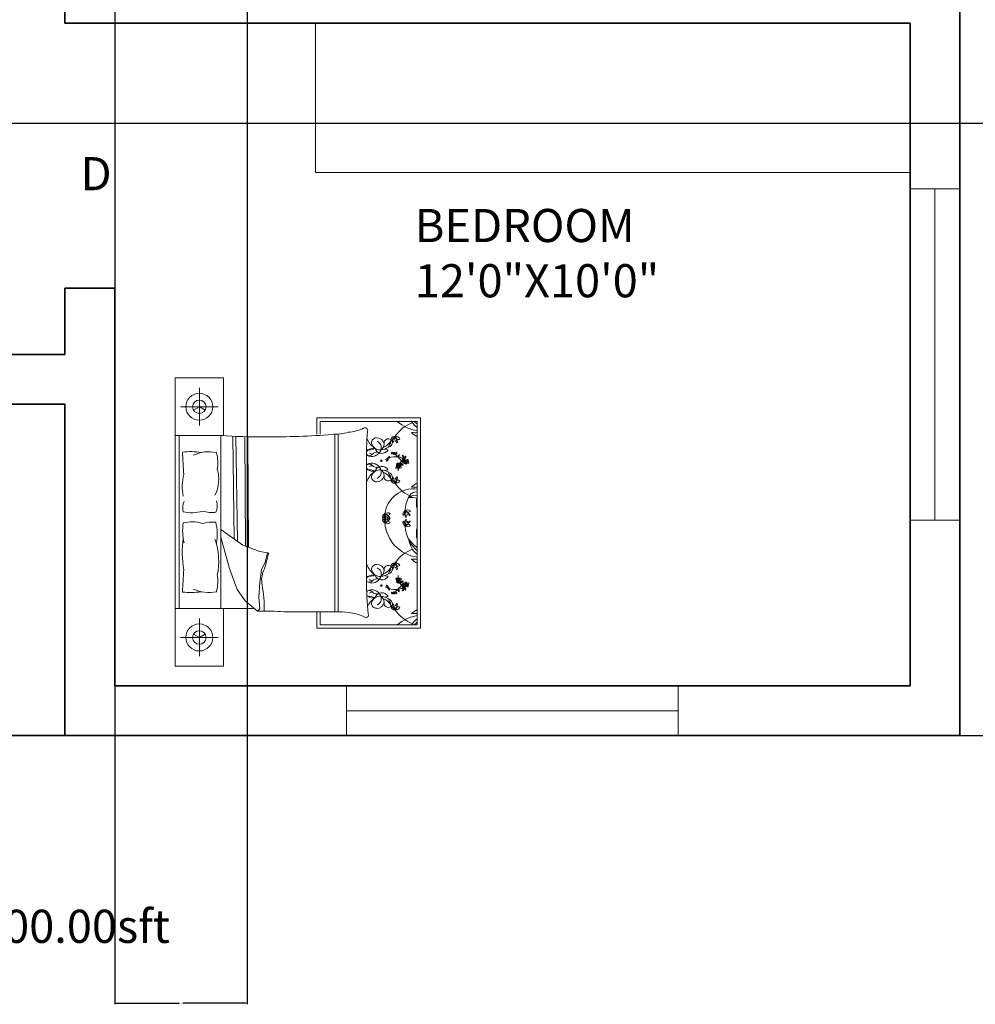
# Model space of a CAD drawing. Units: inches. Extents: x -43 to 1296, y -568 to 542.
# Tile 9 of 14: x 1014 to 1187, y -532 to -354. Entities that reach past the tile are written whole.
import ezdxf

# ---------------------------------------------------------------- set-up
doc = ezdxf.new("R2010")
doc.units = ezdxf.units.IN
doc.header["$MEASUREMENT"] = 0
for name, color, linetype, lineweight in [('A-ANNO-DIMS', 2, 'Continuous', 18), ('A-ANNO-SYMB', 7, 'Continuous', 25), ('A-ANNO-TEXT', 7, 'Continuous', 18), ('A-AREA-IDEN', 7, 'Continuous', 18), ('A-FLOR-CASE', 9, 'Continuous', 18), ('A-FURN', 8, 'Continuous', 13), ('A-GLAZ', 6, 'Continuous', 18), ('A-WALL', 7, 'Continuous', 35)]:
    doc.layers.add(name, color=color, linetype=linetype, lineweight=lineweight)
doc.styles.get("Standard").update_dxf_attribs({"font": 'arial.ttf'})
doc.dimstyles.get("Standard").update_dxf_attribs({"dimtxt": 0.18, "dimasz": 0.18, "dimexe": 0.18, "dimexo": 0.0625, "dimgap": 0.09, "dimtad": 0, "dimtih": 1, "dimtoh": 1, "dimdec": 0, "dimzin": 0, "dimdsep": 46, "dimlunit": 3, "dimtxsty": 'Standard', "dimcen": 0.09, "dimadec": 0, "dimazin": 0, "dimtfac": 1, "dimtdec": 0, "dimtofl": 0, "dimtmove": 0, "dimatfit": 3, "dimfxl": 1, "dimtolj": 1, "dimtzin": 0, "dimarcsym": 0})

# ---------------------------------------------------------------- blocks, each defined once
blk = doc.blocks.new('*D4')
at = {"layer": 'A-ANNO-DIMS', "color": 0, "lineweight": -2, "transparency": 16777216}
for p, q in [((1184.19, -3.76), (1201.25, -3.76)), ((1201.07, -3.94), (1201.07, -240.61)), ((1201.07, -483.58), (1201.07, -246.91)), ((1184.19, -483.76), (1201.25, -483.76))]:
    blk.add_line(p, q, dxfattribs=at)
at = {"layer": 'A-ANNO-DIMS', "color": 0, "transparency": 16777216}
for points in [[(1201.04, -3.94), (1201.1, -3.94), (1201.07, -3.76)], [(1201.04, -483.58), (1201.1, -483.58), (1201.07, -483.76)]]:
    blk.add_solid(points, dxfattribs=at)
at = {"layer": 'Defpoints', "color": 0, "transparency": 16777216}
for p in [(1184.13, -3.76), (1184.13, -483.76), (1201.07, -483.76)]:
    blk.add_point(p, dxfattribs=at)
at = {"layer": 'A-ANNO-DIMS', "color": 0, "transparency": 16777216, "insert": (1201.07, -243.76), "char_height": 6, "attachment_point": 5}
blk.add_mtext("\\A1;40'", dxfattribs=at)
blk = doc.blocks.new('BED-SUITE-52')
for p, q in [((0, 0), (0, 52.23)), ((4.35, 43.59), (4.35, 50.42)), ((7.76, 47), (0.94, 47)), ((25.6, 42.07), (25.6, 44.97)), ((25.6, 44.97), (44.41, 44.97)), ((44.41, 44.97), (44.41, 6.89)), ((26.21, 44.36), (26.21, 42.06)), ((43.81, 44.36), (26.21, 44.36)), ((43.81, 7.5), (43.81, 44.36)), ((0.67, 41.78), (0.67, 10.45)), ((8.25, 10.45), (8.25, 41.78)), ((10.42, 41.64), (10.68, 23.05)), ((10.96, 41.62), (11.23, 22.66)), ((12.6, 41.59), (12.68, 21.76)), ((13.14, 41.6), (13.22, 21.56)), ((28.86, 42.02), (28.86, 9.84)), ((29.51, 42.07), (29.51, 9.84)), ((38.51, 39.22), (37.92, 39.33)), ((34.64, 36.72), (34.64, 15.51)), ((38.51, 35.57), (37.92, 35.45)), ((8.25, 24.79), (12.24, 21.93)), ((9.81, 17.7), (8.25, 23.4)), ((12.24, 21.93), (15.3, 20.77)), ((15.3, 20.77), (16.68, 20.56)), ((16.68, 20.56), (16.25, 18.86)), ((16.25, 18.86), (15.62, 17.49)), ((11.18, 13.89), (9.81, 17.7)), ((15.62, 17.49), (15.3, 15.16)), ((38.51, 16.3), (37.92, 16.41)), ((15.3, 15.16), (15.09, 12.52)), ((12.66, 11.88), (11.18, 13.89)), ((15.09, 12.52), (15.3, 10.4)), ((38.51, 12.65), (37.92, 12.53)), ((14.88, 9.98), (12.66, 11.88)), ((0, 10.45), (14.33, 10.45)), ((15.3, 10.4), (14.88, 9.98)), ((25.6, 6.89), (25.6, 9.85)), ((26.21, 9.85), (26.21, 7.5)), ((4.35, 8.64), (4.35, 1.81)), ((26.21, 7.5), (43.81, 7.5)), ((44.41, 6.89), (25.6, 6.89)), ((7.76, 5.22), (0.94, 5.22))]:
    blk.add_line(p, q)
for points in [[(0, 41.78), (8.7, 41.78), (8.7, 52.23), (0, 52.23)], [(4.35, 47), (3.3, 46.39)], [(4.35, 47), (5.41, 46.39)], [(8.7, 10.45), (8.7, 0), (0, 0)], [(4.35, 5.22), (3.3, 5.83)], [(4.35, 5.22), (5.41, 5.83)]]:
    blk.add_lwpolyline(points)
for points in [[(28.45, 42, 0.056112), (31.32, 42.38, 0.095341), (34.09, 43.12)], [(1.3, 38.78, -0.074897), (4.71, 38.72, 0.472817)], [(4.9, 28.1, -0.14099), (1.42, 27.99, -0.235245)], [(4.9, 25.87, 0.14099), (1.42, 25.97, 0.235245)], [(1.3, 13.45, 0.074897), (4.71, 13.51, -0.472817)], [(19.66, 9.87, 0.001242), (29.57, 9.84, -0.127202), (34.51, 8.8)]]:
    blk.add_lwpolyline(points, format="xyb")
for centre, radius in [((4.35, 47), 2.44), ((4.35, 47), 1.22), ((40.41, 36.2), 0.133), ((41.81, 37.07), 0.133), ((40.41, 15.66), 0.133), ((41.81, 14.79), 0.133), ((4.35, 5.22), 2.44), ((4.35, 5.22), 1.22)]:
    blk.add_circle(centre, radius)
for centre, radius, start, end in [((34.35, 42.72), 0.476, 336.5219, 123.8264), ((45.4, 37.77), 6.82, 111.4092, 145.6135), ((44.73, 49.44), 6.82, 228.1144, 262.255), ((45.64, 46.02), 3.32, 209.8884, 236.5383), ((46.26, 47.22), 4.14, 223.5186, 233.6964), ((14.64, 135.41), 93.84, 266.1, 270.9282), ((18.05, 163.97), 122.41, 269.1145, 274.8735), ((85.43, 38.32), 50.82, 175.2402, 181.8035), ((38.32, 42.79), 3.95, 203.6453, 236.3329), ((36.42, 40.49), 0.882, 88.9462, 185.5144), ((36.55, 40.12), 1.25, 7.1143, 95.0551), ((38.56, 40.41), 0.784, 19.1312, 189.736), ((39.64, 41.08), 0.565, 76.272, 177.0484), ((38.78, 42.23), 1.16, 284.7031, 328.6173), ((40.4, 40.75), 1.08, 125.7657, 194.5347), ((35.12, 42.66), 4.77, 332.8176, 347.4827), ((39.94, 40.89), 0.756, 20.9613, 102.2885), ((40.34, 41.64), 0.57, 181.7131, 301.5367), ((38.48, 40.49), 1.72, 2.0648, 41.1598), ((39.52, 41.13), 0.558, 316.2238, 62.3173), ((44.87, 44.16), 2.77, 221.0454, 247.4453), ((43.38, 51.75), 9.44, 266.3481, 272.5919), ((35.03, 41.34), 2.16, 259.249, 301.1782), ((35.97, 37.49), 2.01, 85.2696, 124.215), ((37.07, 40.76), 1.57, 193.079, 274.7067), ((37.39, 39.86), 1.3, 196.8663, 330.0915), ((36.07, 39.63), 1.21, 338.5779, 68.4181), ((36.27, 40.34), 1.52, 305.9599, 357.6409), ((37.03, 41.99), 2.8, 273.4924, 303.7117), ((36.83, 41.97), 2.47, 288.2955, 328.7386), ((38.32, 40.6), 0.979, 285.6955, 4.031), ((39.62, 39.55), 1.04, 128.4175, 173.8338), ((39.41, 40.57), 0.48, 126.7319, 206.0245), ((39.84, 40.8), 0.0445, 20.2667, 316.2271), ((40.07, 40.56), 0.0411, 52.0591, 168.5166), ((40.11, 40.55), 0.0847, 168.5166, 2.0648), ((-495.72, 9.99), 497.85, 2.8502, 3.3148), ((6.08, 32.13), 6.73, 78.2417, 114.8684), ((0.69, 36.92), 7, 348.9631, 14.8961), ((35.22, 38.66), 0.629, 196.6343, 225.5483), ((35.22, 38.66), 0.629, 127.675, 162.5814), ((35.59, 39.66), 1.66, 240.8249, 340.7178), ((35.09, 38.92), 0.781, 246.1646, 318.4347), ((35.89, 39.91), 1.5, 240.0851, 262.564), ((36.48, 37.7), 1.07, 74.8529, 138.4347), ((36.84, 39.04), 0.324, 254.8529, 12.6959), ((35.97, 37.49), 2.01, 53.6555, 57.2989), ((39.96, 33.62), 4.33, 110.1059, 116.9968), ((37.57, 37.74), 0.839, 336.3901, 344.4871), ((38.48, 37.52), 0.106, 83.9457, 185.6216), ((38.06, 37.62), 0.438, 328.836, 0.8141), ((38.28, 37.49), 0.251, 306.5232, 32.4668), ((38.58, 37.69), 0.106, 112.5583, 214.2343), ((38.51, 37.88), 0.251, 265.7131, 351.6568), ((38.29, 38.02), 0.438, 297.3659, 329.344), ((37.96, 38.39), 0.839, 313.6929, 321.7899), ((38.89, 37.82), 0.274, 115.5379, 168.6744), ((37.96, 38.21), 0.825, 329.344, 349.7412), ((39.96, 33.62), 4.33, 86.1723, 106.4158), ((37.3, 38.02), 1.47, 352.8698, 1.6736), ((39.25, 38.55), 0.103, 125.0752, 284.7644), ((39.41, 38.59), 0.222, 127.3642, 168.4363), ((39.24, 38.77), 0.32, 277.4968, 341.2737), ((39.49, 38.62), 0.127, 88.1325, 178.8919), ((39.75, 38.49), 0.275, 136.3462, 189.6513), ((39.62, 38.78), 0.133, 183.2768, 356.7232), ((39.59, 38.46), 0.115, 189.6513, 312.3208), ((40.03, 38.54), 0.435, 164.2829, 186.9148), ((39.52, 38.54), 0.218, 312.3208, 40.2111), ((39.98, 38.78), 0.309, 201.6382, 274.947), ((39.57, 38.36), 0.404, 42.3896, 66.5724), ((43.64, 41.56), 4.96, 217.9541, 226.8459), ((39.86, 38.6), 0.22, 10.9597, 52.2379), ((40, 38.58), 0.102, 274.947, 37.5263), ((40.34, 38), 0.106, 112.5583, 214.2343), ((40.27, 38.19), 0.251, 265.7131, 351.6568), ((40.05, 38.33), 0.438, 297.3659, 329.344), ((40.07, 35.78), 2.17, 60.7959, 85.244), ((35.46, 32.66), 7.14, 37.8256, 47.7588), ((39.72, 38.7), 0.839, 313.6929, 321.7899), ((40.65, 38.13), 0.274, 115.5379, 168.6744), ((39.72, 38.52), 0.825, 329.344, 349.7412), ((39.06, 38.33), 1.47, 352.8698, 1.6736), ((42.95, 35.55), 2.6, 130.182, 149.456), ((41.13, 38.04), 0.148, 33.0979, 123.1364), ((37.86, 35.94), 3.89, 31.1156, 34.8118), ((40.91, 37.78), 0.402, 2.3172, 70.5201), ((40.72, 37.35), 0.606, 310.9365, 22.7695), ((41.25, 37.68), 0.116, 135.7354, 318.1297), ((41.05, 37.87), 0.154, 315.7354, 31.1156), ((40.92, 37.55), 0.357, 319.3812, 5.5456), ((41.33, 37.68), 0.116, 68.2452, 250.6395), ((41.07, 37.83), 0.346, 352.6008, 57.1845), ((42.3, 35.5), 2.32, 111.7087, 116.2181), ((41.4, 37.91), 0.346, 252.8042, 349.6943), ((41.07, 37.29), 0.369, 331.1838, 51.6792), ((40.07, 35.78), 2.17, 47.5083, 55.9967), ((41.43, 37.93), 0.154, 248.2452, 323.6254), ((41.3, 38.03), 0.402, 291.7087, 3.0299), ((38.43, 40.15), 3.89, 323.6254, 327.3216), ((41.61, 37.93), 0.148, 325.6077, 55.6462), ((42.21, 37.11), 0.419, 121.9501, 165.2442), ((42.06, 37.35), 0.132, 44.3732, 121.9501), ((1.21, 33.9), 6.65, 333.8761, 16.1746), ((35.22, 36.13), 0.629, 134.4517, 156.7144), ((35.22, 36.13), 0.629, 203.2856, 232.325), ((35.59, 35.12), 1.66, 19.2822, 119.1751), ((35.09, 35.86), 0.781, 41.5653, 113.8354), ((35.89, 34.87), 1.5, 97.436, 119.9149), ((36.48, 37.09), 1.07, 221.5653, 285.1471), ((37.39, 34.92), 1.3, 29.9085, 163.1337), ((36.84, 35.74), 0.324, 347.3041, 105.1471), ((35.97, 37.29), 2.01, 302.7011, 306.3445), ((37.27, 37.25), 0.164, 169.5864, 349.5616), ((36.27, 34.44), 1.52, 2.3591, 54.0401), ((37.33, 37.24), 0.101, 349.5616, 167.2949), ((38.51, 37.19), 0.274, 129.5056, 182.6421), ((37.73, 37.82), 0.825, 308.4388, 328.836), ((37.58, 38.49), 1.47, 296.5064, 305.3102), ((40.04, 35.98), 0.103, 125.0752, 284.7644), ((40.2, 36.02), 0.222, 93.635, 168.4363), ((40.21, 37.22), 0.606, 253.6301, 325.4631), ((40.38, 36.38), 0.429, 82.0748, 142.6895), ((40.33, 36.97), 0.441, 228.342, 274.9894), ((40.17, 36.37), 0.13, 138.2946, 276.2474), ((40.03, 36.19), 0.32, 277.4968, 341.2737), ((40.22, 36.35), 0.181, 358.5719, 143.8954), ((40.28, 36.04), 0.127, 88.1325, 178.8919), ((40.33, 36.49), 0.183, 208.8493, 269.9355), ((40.17, 36.45), 0.209, 274.2123, 318.1587), ((40.54, 35.91), 0.275, 136.3462, 189.6513), ((40.38, 35.88), 0.115, 189.6513, 312.3208), ((42.95, 35.55), 2.6, 175.2415, 182.8929), ((40.34, 36.89), 0.369, 273.8774, 357.1501), ((40.82, 35.96), 0.435, 164.2829, 186.9148), ((40.81, 36.24), 0.419, 121.9501, 165.2442), ((40.49, 37.15), 0.357, 262.0748, 308.2393), ((40.31, 35.96), 0.218, 312.3208, 40.2111), ((40.77, 36.2), 0.309, 201.6382, 274.947), ((40.52, 36.4), 0.0881, 262.868, 7.094), ((40.36, 35.78), 0.404, 42.3896, 66.5724), ((40.51, 36.47), 0.262, 278.5614, 22.5914), ((40.65, 36.02), 0.22, 10.9597, 118.7804), ((42.95, 35.55), 2.6, 156.1523, 156.9499), ((40.66, 36.48), 0.132, 44.3732, 121.9501), ((41.06, 36.79), 0.369, 181.4625, 249.4747), ((41, 37.08), 0.357, 215.1128, 261.2773), ((41.29, 37.06), 0.606, 197.889, 269.722), ((40.79, 36), 0.102, 274.947, 37.5263), ((41.1, 36.85), 0.441, 248.3627, 295.0101), ((40.88, 36.3), 0.429, 20.6625, 81.2773), ((41.52, 37.04), 0.429, 139.3812, 199.9959), ((41, 37.31), 0.441, 285.6484, 332.2957), ((41.44, 36.85), 0.103, 125.0752, 284.7644), ((41.6, 36.89), 0.222, 93.635, 168.4363), ((41.57, 37.24), 0.13, 138.2946, 276.2474), ((41.43, 37.06), 0.32, 277.4968, 341.2737), ((41.62, 37.22), 0.181, 358.5719, 143.8954), ((41.68, 36.91), 0.127, 88.1325, 178.8919), ((41.73, 37.36), 0.183, 208.8493, 269.9355), ((41.57, 37.32), 0.209, 274.2123, 318.1587), ((41.94, 36.78), 0.275, 136.3462, 189.6513), ((41.78, 36.75), 0.115, 189.6513, 312.3208), ((42.22, 36.83), 0.435, 164.2829, 186.9148), ((41.71, 36.83), 0.218, 312.3208, 40.2111), ((42.17, 37.07), 0.309, 201.6382, 274.947), ((41.92, 37.27), 0.0881, 262.868, 7.094), ((41.76, 36.65), 0.404, 42.3896, 66.5724), ((41.91, 37.34), 0.262, 278.5614, 22.5914), ((42.06, 36.89), 0.22, 10.9597, 118.7804), ((42.19, 36.87), 0.102, 274.947, 37.5263), ((10.44, 32.58), 9.18, 166.3427, 191.1841), ((35.03, 33.45), 2.16, 58.8218, 100.2867), ((38.32, 32), 3.95, 123.6671, 158.5059), ((35.97, 37.29), 2.01, 235.785, 274.7304), ((37.07, 34.03), 1.57, 85.2933, 166.921), ((36.42, 34.3), 0.882, 174.4856, 271.0538), ((36.55, 34.66), 1.25, 264.9449, 352.8857), ((36.07, 35.15), 1.21, 291.5819, 21.4221), ((37.03, 32.8), 2.8, 56.2883, 86.5076), ((36.83, 32.82), 2.47, 31.2614, 71.7045), ((38.56, 34.37), 0.784, 170.264, 340.8688), ((39.62, 35.24), 1.04, 186.1662, 231.5825), ((38.32, 34.18), 0.979, 355.969, 74.3045), ((39.41, 34.21), 0.48, 153.9755, 233.2681), ((40.4, 34.03), 1.08, 165.4653, 234.2343), ((35.12, 32.13), 4.77, 12.5173, 27.1824), ((38.48, 34.29), 1.72, 318.8402, 357.9352), ((39.52, 33.65), 0.558, 297.6827, 43.7762), ((39.86, 33.99), 0.0738, 43.7762, 339.7183), ((40.11, 34.24), 0.0847, 357.9352, 191.4834), ((40.07, 34.23), 0.0411, 191.4834, 307.9409), ((43.15, 26.86), 5.28, 82.8636, 171.8197), ((39.64, 33.71), 0.565, 182.9516, 283.728), ((38.78, 32.55), 1.16, 31.3827, 75.2969), ((40.34, 33.14), 0.57, 58.4633, 178.2869), ((39.94, 33.9), 0.756, 257.7115, 339.0387), ((45.4, 37.01), 6.82, 214.3865, 248.5908), ((44.87, 30.63), 2.77, 112.5547, 138.9546), ((43.38, 23.03), 9.44, 87.4081, 93.6519), ((48.38, 27.61), 6.82, 152.5854, 175.5377), ((43.52, 30.35), 1.22, 76.3898, 169.0739), ((43.35, 29.43), 1.55, 72.8609, 131.9049), ((42.67, 27.55), 3.05, 68.117, 96.6195), ((47.4, 29.51), 3.75, 162.9798, 196.4569), ((3.91, 28.71), 2.58, 153.3437, 196.1026), ((4.81, 29.06), 2.77, 335.0183, 18.5407), ((49.33, 28.03), 5.55, 174.3643, 175.6213), ((6.65, 34.26), 6.4, 254.1707, 275.9871), ((38.09, 27.07), 0.565, 106.1963, 206.9726), ((38.09, 26.53), 0.565, 153.0274, 253.8037), ((36.76, 27.64), 1.16, 314.6273, 358.5415), ((36.76, 25.96), 1.16, 1.4585, 45.3727), ((38.91, 27.17), 1.08, 155.6899, 224.4589), ((38.91, 26.43), 1.08, 135.5411, 204.3101), ((38.44, 27.05), 0.756, 50.8855, 132.2127), ((38.41, 27.91), 0.57, 211.6373, 331.4609), ((37.95, 27.06), 0.558, 346.148, 92.2415), ((37.37, 25.98), 1.72, 31.989, 71.0841), ((33.38, 26.19), 4.77, 2.7418, 17.407), ((33.38, 27.42), 4.77, 342.593, 357.2582), ((38.39, 26.93), 0.0445, 50.1909, 346.0209), ((38.76, 26.85), 0.0847, 198.4408, 31.989), ((38.72, 26.84), 0.0411, 81.9833, 198.4408), ((38.76, 26.75), 0.0847, 328.011, 161.5592), ((38.72, 26.77), 0.0411, 161.5592, 278.0167), ((41.74, 27.59), 0.565, 106.1963, 206.9726), ((40.42, 28.17), 1.16, 314.6273, 358.5415), ((42.56, 27.69), 1.08, 155.6899, 224.4589), ((42.09, 27.58), 0.756, 50.8855, 132.2127), ((42.07, 28.44), 0.57, 211.6373, 331.4609), ((41.02, 26.51), 1.72, 31.989, 71.0841), ((37.03, 26.71), 4.77, 2.7418, 17.407), ((41.6, 27.58), 0.558, 346.148, 92.2415), ((42.05, 27.46), 0.0445, 50.1909, 346.0209), ((42.41, 27.37), 0.0847, 198.4408, 31.989), ((42.37, 27.36), 0.0411, 81.9833, 198.4408), ((53.13, 25.11), 9.91, 160.0972, 160.2783), ((10.63, 24.6), 9.31, 171.5249, 193.96), ((6.65, 19.71), 6.4, 84.0129, 105.8293), ((-1.63, 23.91), 9.21, 349.8617, 13.6238), ((37.37, 27.62), 1.72, 288.9159, 328.011), ((37.95, 26.55), 0.558, 267.7585, 13.852), ((38.41, 25.69), 0.57, 28.5391, 148.3627), ((38.44, 26.55), 0.756, 227.7873, 309.1145), ((44.73, 26.52), 6.82, 184.4623, 262.255), ((38.42, 26.66), 0.0738, 13.852, 309.9245), ((41.74, 26.01), 0.565, 153.0274, 253.8037), ((40.42, 25.44), 1.16, 1.4585, 45.3727), ((42.56, 25.91), 1.08, 135.5411, 204.3101), ((37.03, 26.89), 4.77, 342.593, 357.2582), ((41.02, 27.1), 1.72, 288.9159, 328.011), ((41.6, 26.02), 0.558, 267.7585, 13.852), ((42.07, 25.17), 0.57, 28.5391, 148.3627), ((42.09, 26.03), 0.756, 227.7873, 309.1145), ((48.38, 26), 6.82, 184.4623, 207.4146), ((42.07, 26.14), 0.0738, 13.852, 309.9245), ((42.41, 26.23), 0.0847, 328.011, 161.5592), ((42.37, 26.24), 0.0411, 161.5592, 278.0167), ((47.4, 24.09), 3.75, 163.5431, 197.0202), ((49.33, 25.58), 5.55, 184.3787, 185.6357), ((53.13, 28.5), 9.91, 199.7217, 199.9028), ((20.2, 20.6), 18.94, 172.2196, 189.497), ((-4.28, 18.99), 12.14, 348.0397, 19.2615), ((45.64, 23.1), 3.32, 181.272, 236.5383), ((47.43, 26.47), 6.16, 214.0123, 234.053), ((46.26, 24.29), 4.14, 197.8504, 233.6964), ((-3.06, 24.18), 20.25, 340.1194, 349.3383), ((16.72, 20.44), 0.126, 358.8623, 109.7536), ((45.4, 14.85), 6.82, 111.4092, 145.6135), ((38.32, 19.87), 3.95, 201.4941, 236.3329), ((36.42, 17.56), 0.882, 88.9462, 185.5144), ((36.55, 17.2), 1.25, 7.1143, 95.0551), ((36.07, 16.71), 1.21, 338.5779, 68.4181), ((38.56, 17.49), 0.784, 19.1312, 189.736), ((39.41, 17.65), 0.48, 126.7319, 206.0245), ((39.64, 18.15), 0.565, 76.272, 177.0484), ((38.78, 19.31), 1.16, 284.7031, 328.6173), ((40.4, 17.83), 1.08, 125.7657, 194.5347), ((35.12, 19.74), 4.77, 332.8176, 347.4827), ((39.94, 17.96), 0.756, 20.9613, 102.2885), ((39.52, 18.21), 0.558, 316.2238, 62.3173), ((38.48, 17.57), 1.72, 2.0648, 41.1598), ((40.34, 18.72), 0.57, 181.7131, 301.5367), ((39.84, 17.88), 0.0445, 20.2667, 316.2271), ((43.38, 28.83), 9.44, 266.3481, 272.5919), ((44.87, 21.24), 2.77, 221.0454, 247.4453), ((-495.72, 42.23), 497.85, 356.6852, 357.1498), ((0.69, 15.31), 7, 345.1039, 11.0369), ((19.88, 15.58), 4.25, 156.2616, 191.3392), ((35.03, 18.42), 2.16, 259.7133, 301.1782), ((35.22, 15.74), 0.629, 127.675, 156.7144), ((35.59, 16.74), 1.66, 240.8249, 340.7178), ((35.97, 14.57), 2.01, 85.2696, 124.215), ((37.07, 17.84), 1.57, 193.079, 274.7067), ((37.39, 16.94), 1.3, 196.8663, 330.0915), ((36.84, 16.12), 0.324, 254.8529, 12.6959), ((35.97, 14.57), 2.01, 53.6555, 57.2989), ((36.27, 17.42), 1.52, 305.9599, 357.6409), ((37.03, 19.07), 2.8, 273.4924, 303.7117), ((36.83, 19.04), 2.47, 288.2955, 328.7386), ((38.32, 17.68), 0.979, 285.6955, 4.031), ((39.62, 16.62), 1.04, 128.4175, 173.8338), ((40.07, 17.64), 0.0411, 52.0591, 168.5166), ((40.11, 17.63), 0.0847, 168.5166, 2.0648), ((40.38, 15.98), 0.115, 47.6792, 170.3487), ((42.95, 16.31), 2.6, 177.1071, 184.7585), ((40.31, 15.9), 0.218, 319.7889, 47.6792), ((-3.62, 10.87), 19.71, 357.4519, 11.3392), ((89, 14.89), 54.37, 179.3433, 185.6887), ((35.22, 15.74), 0.629, 203.229, 225.5483), ((35.09, 16), 0.781, 246.1646, 318.4347), ((35.89, 16.99), 1.5, 240.0851, 262.564), ((36.48, 14.77), 1.07, 74.8529, 138.4347), ((37.27, 14.61), 0.164, 10.4384, 190.4136), ((37.33, 14.62), 0.101, 192.7051, 10.4384), ((39.96, 18.24), 4.33, 243.0032, 249.8941), ((37.73, 14.04), 0.825, 31.164, 51.5612), ((38.51, 14.68), 0.274, 177.3579, 230.4944), ((37.58, 13.37), 1.47, 54.6898, 63.4936), ((37.57, 14.13), 0.839, 15.5129, 23.6099), ((38.48, 14.34), 0.106, 174.3784, 276.0543), ((38.28, 14.37), 0.251, 327.5332, 53.4768), ((38.06, 14.24), 0.438, 359.1859, 31.164), ((40.04, 15.89), 0.103, 75.2356, 234.9248), ((40.2, 15.85), 0.222, 191.5637, 266.365), ((40.17, 15.5), 0.13, 83.7526, 221.7054), ((40.33, 14.9), 0.441, 85.0106, 131.658), ((40.21, 14.64), 0.606, 34.5369, 106.3699), ((40.38, 15.49), 0.429, 217.3105, 277.9252), ((40.03, 15.67), 0.32, 18.7263, 82.5032), ((40.22, 15.52), 0.181, 216.1046, 1.4281), ((40.28, 15.82), 0.127, 181.1081, 271.8675), ((40.33, 15.37), 0.183, 90.0645, 151.1507), ((40.17, 15.42), 0.209, 41.8413, 85.7877), ((35.46, 19.21), 7.14, 312.2412, 322.1744), ((40.54, 15.95), 0.275, 170.3487, 223.6538), ((40.34, 14.97), 0.369, 2.8499, 86.1226), ((40.82, 15.9), 0.435, 173.0852, 195.7171), ((40.81, 15.63), 0.419, 194.7558, 238.0499), ((40.49, 14.71), 0.357, 51.7607, 97.9252), ((40.77, 15.66), 0.309, 85.053, 158.3618), ((40.52, 15.47), 0.0881, 352.906, 97.132), ((40.36, 16.08), 0.404, 293.4276, 317.6104), ((40.65, 15.84), 0.22, 241.2196, 349.0403), ((40.51, 15.39), 0.262, 337.4086, 81.4386), ((42.95, 16.31), 2.6, 203.0501, 203.8477), ((40.66, 15.38), 0.132, 238.0499, 315.6268), ((41.06, 15.07), 0.369, 110.5253, 178.5375), ((41.29, 14.8), 0.606, 90.278, 162.111), ((41, 14.78), 0.357, 98.7227, 144.8872), ((42.95, 16.31), 2.6, 210.544, 229.818), ((40.79, 15.86), 0.102, 322.4737, 85.053), ((41.1, 15.01), 0.441, 64.9899, 111.6373), ((40.88, 15.56), 0.429, 278.7227, 339.3375), ((41.52, 14.83), 0.429, 160.0041, 220.6188), ((40.72, 14.52), 0.606, 337.2305, 49.0635), ((41, 14.55), 0.441, 27.7043, 74.3516), ((41.25, 14.18), 0.116, 41.8703, 224.2646), ((40.92, 14.32), 0.357, 354.4544, 40.6188), ((41.33, 14.18), 0.116, 109.3605, 291.7548), ((42.3, 16.36), 2.32, 243.7819, 248.2913), ((41.07, 14.58), 0.369, 308.3208, 28.8162), ((40.07, 16.09), 2.17, 304.0033, 312.4917), ((41.4, 13.96), 0.346, 10.3057, 107.1958), ((41.44, 15.02), 0.103, 75.2356, 234.9248), ((41.6, 14.98), 0.222, 191.5637, 266.365), ((41.57, 14.63), 0.13, 83.7526, 221.7054), ((41.43, 14.8), 0.32, 18.7263, 82.5032), ((41.62, 14.65), 0.181, 216.1046, 1.4281), ((41.68, 14.95), 0.127, 181.1081, 271.8675), ((41.73, 14.5), 0.183, 90.0645, 151.1507), ((41.57, 14.55), 0.209, 41.8413, 85.7877), ((41.94, 15.08), 0.275, 170.3487, 223.6538), ((41.78, 15.11), 0.115, 47.6792, 170.3487), ((42.22, 15.03), 0.435, 173.0852, 195.7171), ((42.21, 14.76), 0.419, 194.7558, 238.0499), ((41.71, 15.03), 0.218, 319.7889, 47.6792), ((42.17, 14.79), 0.309, 85.053, 158.3618), ((41.92, 14.6), 0.0881, 352.906, 97.132), ((41.76, 15.21), 0.404, 293.4276, 317.6104), ((42.06, 14.97), 0.22, 241.2196, 349.0403), ((41.91, 14.52), 0.262, 337.4086, 81.4386), ((42.06, 14.51), 0.132, 238.0499, 315.6268), ((42.19, 14.99), 0.102, 322.4737, 85.053), ((6.08, 20.1), 6.73, 245.1316, 281.7583), ((35.22, 13.2), 0.629, 134.4517, 153.558), ((35.22, 13.2), 0.629, 210.0293, 232.325), ((35.03, 10.52), 2.16, 58.8218, 99.1554), ((35.59, 12.2), 1.66, 19.2822, 119.1751), ((35.09, 12.94), 0.781, 41.5653, 113.8354), ((35.97, 14.37), 2.01, 235.785, 274.7304), ((35.89, 11.95), 1.5, 97.436, 119.9149), ((37.07, 11.11), 1.57, 85.2933, 166.921), ((36.48, 14.17), 1.07, 221.5653, 285.1471), ((37.39, 12), 1.3, 29.9085, 163.1337), ((36.07, 12.23), 1.21, 291.5819, 21.4221), ((36.84, 12.82), 0.324, 347.3041, 105.1471), ((35.97, 14.37), 2.01, 302.7011, 306.3445), ((36.27, 11.52), 1.52, 2.3591, 54.0401), ((37.03, 9.87), 2.8, 56.2883, 86.5076), ((38.58, 14.18), 0.106, 145.7657, 247.4417), ((38.51, 13.99), 0.251, 8.3432, 94.2869), ((38.29, 13.85), 0.438, 30.656, 62.6341), ((37.96, 13.47), 0.839, 38.2101, 46.3071), ((38.89, 14.04), 0.274, 191.3256, 244.4621), ((37.96, 13.65), 0.825, 10.2588, 30.656), ((39.96, 18.24), 4.33, 253.5842, 273.8277), ((37.3, 13.84), 1.47, 358.3264, 7.1302), ((39.25, 13.31), 0.103, 75.2356, 234.9248), ((39.41, 13.27), 0.222, 191.5637, 232.6358), ((39.24, 13.09), 0.32, 18.7263, 82.5032), ((39.49, 13.24), 0.127, 181.1081, 271.8675), ((39.75, 13.37), 0.275, 170.3487, 223.6538), ((39.59, 13.4), 0.115, 47.6792, 170.3487), ((39.62, 13.08), 0.133, 3.2768, 176.7232), ((40.03, 13.32), 0.435, 173.0852, 195.7171), ((39.52, 13.33), 0.218, 319.7889, 47.6792), ((39.98, 13.08), 0.309, 85.053, 158.3618), ((43.64, 10.31), 4.96, 133.1541, 142.0459), ((39.57, 13.5), 0.404, 293.4276, 317.6104), ((39.86, 13.27), 0.22, 307.7621, 349.0403), ((40, 13.29), 0.102, 322.4737, 85.053), ((40.34, 13.86), 0.106, 145.7657, 247.4417), ((40.07, 16.09), 2.17, 274.756, 299.2041), ((40.27, 13.67), 0.251, 8.3432, 94.2869), ((40.05, 13.54), 0.438, 30.656, 62.6341), ((39.72, 13.16), 0.839, 38.2101, 46.3071), ((40.65, 13.73), 0.274, 191.3256, 244.4621), ((39.72, 13.34), 0.825, 10.2588, 30.656), ((39.06, 13.53), 1.47, 358.3264, 7.1302), ((40.91, 14.08), 0.402, 289.4799, 357.6828), ((37.86, 15.92), 3.89, 325.1882, 328.8844), ((41.13, 13.83), 0.148, 236.8636, 326.9021), ((41.05, 13.99), 0.154, 328.8844, 44.2646), ((41.07, 14.04), 0.346, 302.8155, 7.3992), ((41.43, 13.93), 0.154, 36.3746, 111.7548), ((41.3, 13.83), 0.402, 356.9701, 68.2913), ((38.43, 11.71), 3.89, 32.6784, 36.3746), ((41.61, 13.94), 0.148, 304.3538, 34.3923), ((38.32, 9.07), 3.95, 123.6671, 153.2997), ((36.42, 11.38), 0.882, 174.4856, 271.0538), ((36.55, 11.74), 1.25, 264.9449, 352.8857), ((36.83, 9.9), 2.47, 31.2614, 71.7045), ((38.56, 11.45), 0.784, 170.264, 340.8688), ((38.32, 11.26), 0.979, 355.969, 74.3045), ((39.62, 12.32), 1.04, 186.1662, 231.5825), ((39.41, 11.29), 0.48, 153.9755, 233.2681), ((38.78, 9.63), 1.16, 31.3827, 75.2969), ((39.64, 10.79), 0.565, 182.9516, 283.728), ((40.4, 11.11), 1.08, 165.4653, 234.2343), ((35.12, 9.2), 4.77, 12.5173, 27.1824), ((38.48, 11.37), 1.72, 318.8402, 357.9352), ((39.52, 10.73), 0.558, 297.6827, 43.7762), ((40.34, 10.22), 0.57, 58.4633, 178.2869), ((39.94, 10.98), 0.756, 257.7115, 339.0387), ((39.86, 11.07), 0.0738, 43.7762, 339.7183), ((40.11, 11.31), 0.0847, 357.9352, 191.4834), ((40.07, 11.31), 0.0411, 191.4834, 307.9409), ((16.18, -37.91), 47.9, 85.8294, 91.553), ((34.48, 9.28), 0.482, 273.98, 27.3412), ((45.4, 14.09), 6.82, 214.3865, 248.5908), ((44.73, 2.42), 6.82, 97.745, 131.8856), ((44.87, 7.7), 2.77, 112.5547, 138.9546), ((43.38, 0.11), 9.44, 87.4081, 93.6519), ((45.64, 5.84), 3.32, 123.4617, 150.1116), ((46.26, 4.65), 4.14, 126.3036, 136.4814)]:
    blk.add_arc(centre, radius, start, end)
blk = doc.blocks.new('WIN-60x9')
for p, q in [((0, 60), (0, 0)), ((9, 60), (0, 60)), ((4.5, 60), (4.5, 0)), ((9, 0), (9, 60)), ((0, 0), (9, 0))]:
    blk.add_line(p, q)
blk = doc.blocks.new('*D79')
at = {"layer": 'A-ANNO-DIMS', "color": 0, "lineweight": -2, "transparency": 16777216}
for p, q in [((1260.71, -372.83), (1295.51, -372.83)), ((1295.33, -373.01), (1295.33, -428.11)), ((1295.33, -483.58), (1295.33, -428.48)), ((1184.19, -483.76), (1295.51, -483.76))]:
    blk.add_line(p, q, dxfattribs=at)
at = {"layer": 'A-ANNO-DIMS', "color": 0, "transparency": 16777216}
for points in [[(1295.3, -373.01), (1295.36, -373.01), (1295.33, -372.83)], [(1295.3, -483.58), (1295.36, -483.58), (1295.33, -483.76)]]:
    blk.add_solid(points, dxfattribs=at)
at = {"layer": 'Defpoints', "color": 0, "transparency": 16777216}
for p in [(1260.65, -372.83), (1295.33, -372.83), (1184.13, -483.76)]:
    blk.add_point(p, dxfattribs=at)
at = {"layer": 'A-ANNO-DIMS', "color": 0, "transparency": 16777216, "insert": (1295.33, -428.3), "char_height": 0.18, "attachment_point": 5}
blk.add_mtext('\\A1;9\'-3"', dxfattribs=at)
blk = doc.blocks.new('*D83')
at = {"layer": 'A-ANNO-DIMS', "color": 0, "lineweight": -2, "transparency": 16777216}
for p, q in [((1031.13, -225.82), (1031.13, -532.44)), ((1055.13, -225.82), (1055.13, -532.44)), ((1031.31, -532.26), (1042.8, -532.26)), ((1054.95, -532.26), (1043.46, -532.26))]:
    blk.add_line(p, q, dxfattribs=at)
at = {"layer": 'A-ANNO-DIMS', "color": 0, "transparency": 16777216}
for points in [[(1031.31, -532.23), (1031.31, -532.29), (1031.13, -532.26)], [(1054.95, -532.23), (1054.95, -532.29), (1055.13, -532.26)]]:
    blk.add_solid(points, dxfattribs=at)
at = {"layer": 'Defpoints', "color": 0, "transparency": 16777216}
for p in [(1031.13, -225.76), (1055.13, -225.76), (1055.13, -532.26)]:
    blk.add_point(p, dxfattribs=at)
at = {"layer": 'A-ANNO-DIMS', "color": 0, "transparency": 16777216, "insert": (1043.13, -532.26), "char_height": 0.18, "attachment_point": 5}
blk.add_mtext('\\A1;2\'-0"', dxfattribs=at)

msp = doc.modelspace()

# ---------------------------------------------------------------- linework, layer by layer
at = {"layer": 'A-ANNO-SYMB'}
msp.add_line((795.05, -372.83), (1260.65, -372.83), dxfattribs=at)
at = {"layer": 'A-FLOR-CASE'}
for p, q in [((1067.5, -354.76), (1067.5, -381.76)), ((1067.5, -381.76), (1175.13, -381.76))]:
    msp.add_line(p, q, dxfattribs=at)
at = {"layer": 'A-WALL'}
for p, q in [((1184.13, -3.76), (1184.13, -483.76)), ((1022.13, -270.76), (1022.13, -354.76)), ((1022.13, -354.76), (1175.13, -354.76)), ((1175.13, -354.76), (1175.13, -474.76)), ((1022.13, -402.76), (1022.13, -414.76)), ((1022.13, -402.76), (1031.13, -402.76)), ((1031.13, -402.76), (1031.13, -474.76)), ((875.13, -414.76), (1022.13, -414.76)), ((875.13, -423.76), (1022.13, -423.76)), ((1022.13, -423.76), (1022.13, -483.76)), ((1031.13, -474.76), (1175.13, -474.76)), ((824.13, -483.76), (1184.13, -483.76))]:
    msp.add_line(p, q, dxfattribs=at)

# ---------------------------------------------------------------- block references
at = {"layer": 'A-FURN'}
msp.add_blockref('BED-SUITE-52', (1042.11, -471.22), dxfattribs=at)
at = {"layer": 'A-GLAZ'}
msp.add_blockref('WIN-60x9', (1175.13, -444.76), dxfattribs=at)
at = {"layer": 'A-GLAZ', "rotation": 270.0000000000002}
msp.add_blockref('WIN-60x9', (1073.13, -474.76), dxfattribs=at)

# ---------------------------------------------------------------- texts
at = {"layer": 'A-ANNO-TEXT', "insert": (1024.95, -379), "char_height": 6, "attachment_point": 1}
msp.add_mtext('D', dxfattribs=at)
at = {"layer": 'A-AREA-IDEN', "insert": (1085.46, -388.39), "char_height": 6, "attachment_point": 1}
msp.add_mtext('BEDROOM\\P12\'0"X10\'0"', dxfattribs=at)
at = {"layer": 'A-AREA-IDEN', "insert": (937.24, -515.31), "char_height": 6, "attachment_point": 1}
msp.add_mtext_dynamic_manual_height_columns('GROUND FLOOR:1200.00sft', width=119.732, gutter_width=1, heights=[15.32], dxfattribs=at)

# ---------------------------------------------------------------- dimensions: what is measured, and where the dimension line sits
at = {"layer": 'A-ANNO-DIMS'}
for base, p1, p2, override, picture, middle in [((1201.07, -483.76), (1184.13, -3.76), (1184.13, -483.76), {"dimtxt": 6, "dimclrd": 0, "dimclre": 0, "dimclrt": 0}, '*D4', (1201.07, -243.76)), ((1295.33, -372.83), (1184.13, -483.76), (1260.65, -372.83), {"dimdec": 1, "dimlfac": 1, "dimrnd": 0, "dimzin": 1, "dimdsep": 46, "dimlunit": 4, "dimfrac": 2}, '*D79', (1295.33, -428.3))]:
    dim = msp.add_linear_dim(base=base, p1=p1, p2=p2, angle=90, dimstyle='Standard', override=override, dxfattribs=at)
    dim.commit()
    dim.dimension.update_dxf_attribs({"geometry": picture, "text_midpoint": middle})
dim = msp.add_linear_dim(base=(1055.13, -532.26), p1=(1031.13, -225.76), p2=(1055.13, -225.76), dimstyle='Standard', override={"dimdec": 1, "dimlfac": 1, "dimrnd": 0, "dimzin": 1, "dimdsep": 46, "dimlunit": 4, "dimfrac": 2}, dxfattribs=at)
dim.commit()
dim.dimension.update_dxf_attribs({"geometry": '*D83', "text_midpoint": (1043.13, -532.26)})

doc.saveas('drawing.dxf')
